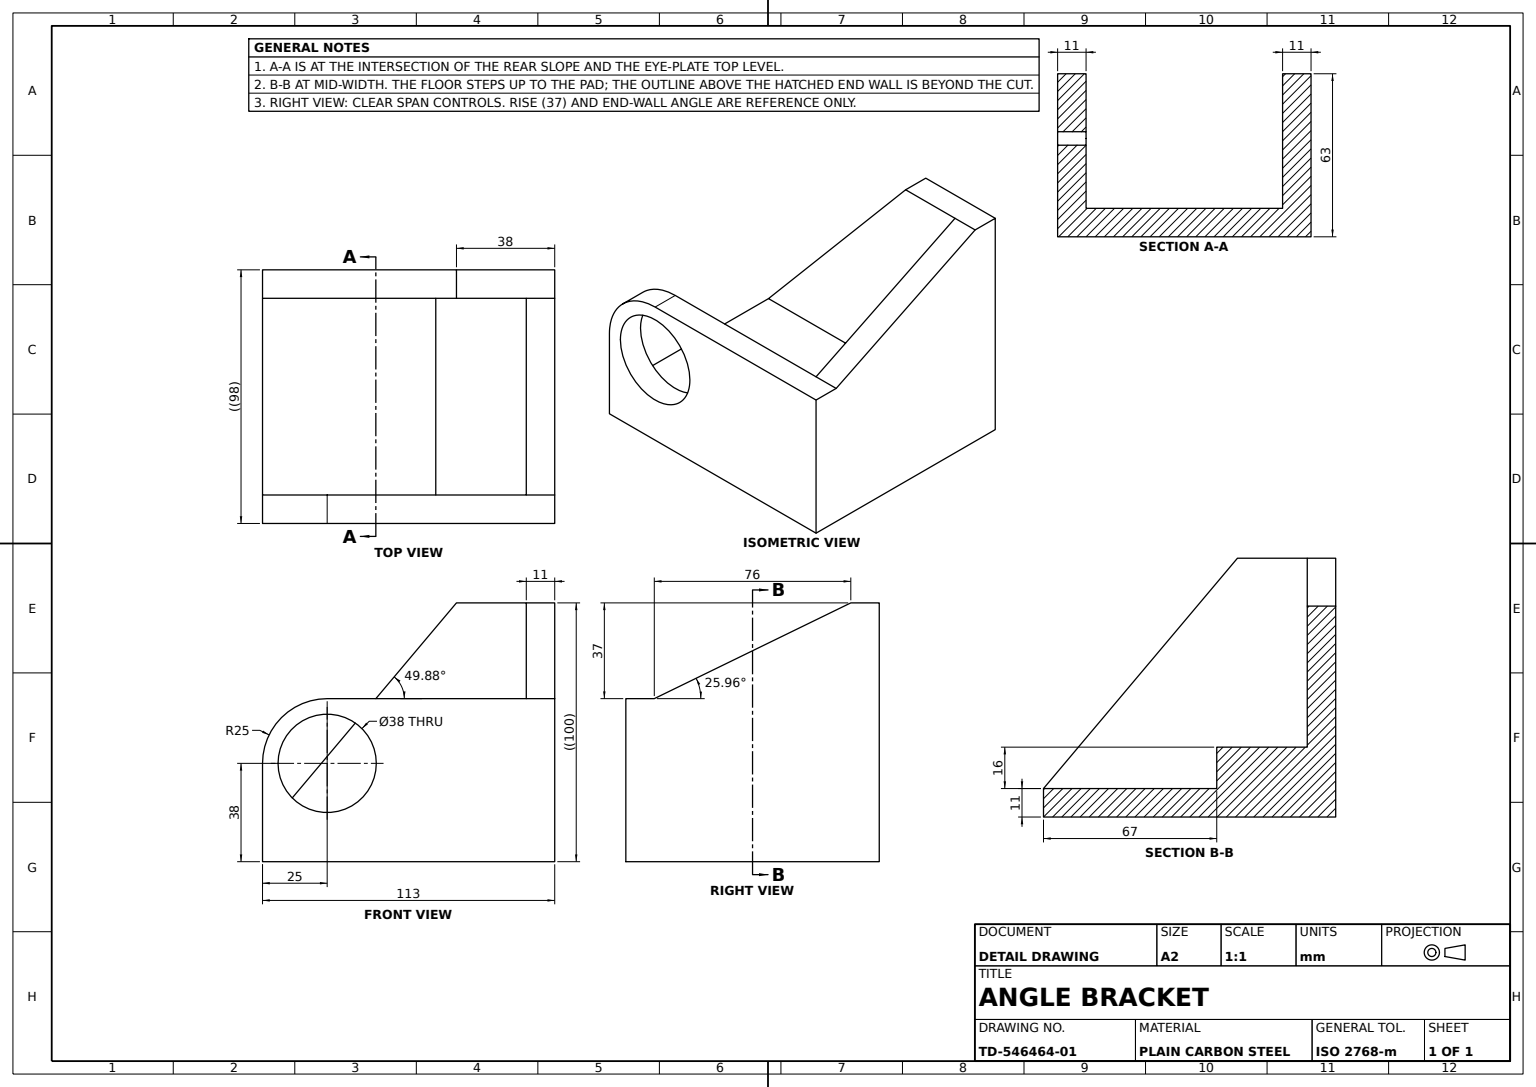
from build123d import *

# Parameters (mm, degrees)
EYE_PLATE_11MM_DEPTH    = 11
FLOOR_PLATE_11MM_DEPTH  = 11
SIDE_WALL_11MM_DEPTH    = 11
INCLINED_WEB_PROFILE_W  = 102
INCLINED_WEB_PROFILE_H  = 76
INCLINED_WEB_11MM_DEPTH = 11
END_CAP_PROFILE_W       = 35
END_CAP_PROFILE_H       = 76
END_CAP_16MM_DEPTH      = 16
PIVOT_BORE_PROFILE_R    = 19
PIVOT_BORE_38_DEPTH     = 11


with BuildPart() as part:
    # Eye Plate Profile → Eye Plate 11mm (new body)
    with BuildSketch(Plane.XY):
        with BuildLine():
            Line((0, 0), (113, 0))
            Line((113, 0), (113, 63))
            Line((113, 63), (25, 63))
            ThreePointArc((25, 63), (7.32233047, 55.67766953), (0, 38))
            Line((0, 38), (0, 0))
        make_face()
    extrude(amount=EYE_PLATE_11MM_DEPTH)

    # Floor Plate Profile → Floor Plate 11mm (add)
    with BuildSketch(Plane(origin=(113, 0, 0), x_dir=(0, 0, -1), z_dir=(1, 0, 0))):
        Polygon((0, 0), (76, 0), (76, 100), (0, 63), align=None)
    extrude(amount=-FLOOR_PLATE_11MM_DEPTH)

    # Side Wall Profile → Side Wall 11mm (add)
    with BuildSketch(Plane(origin=(0, 0, -76), x_dir=(-1, 0, 0), z_dir=(0, 0, -1))):
        Polygon((-113, 0), (0, 0), (0, 11), (-75, 100), (-113, 100), align=None)
    extrude(amount=SIDE_WALL_11MM_DEPTH)

    # Inclined Web Profile → Inclined Web 11mm (add)
    with BuildSketch(Plane.XZ):
        with Locations((51, -38)):
            Rectangle(INCLINED_WEB_PROFILE_W, INCLINED_WEB_PROFILE_H)
    extrude(amount=-INCLINED_WEB_11MM_DEPTH)

    # End Cap Profile → End Cap 16mm (add)
    with BuildSketch(Plane(origin=(0, 11, 0), x_dir=(1, 0, 0), z_dir=(0, 1, 0))):
        with Locations((84.5, 38)):
            Rectangle(END_CAP_PROFILE_W, END_CAP_PROFILE_H)
    extrude(amount=END_CAP_16MM_DEPTH)

    # Pivot Bore Profile → Pivot Bore Ø38 (cut)
    with BuildSketch(Plane.XY.offset(11)):
        with Locations((25, 38)):
            Circle(PIVOT_BORE_PROFILE_R)
    extrude(amount=-PIVOT_BORE_38_DEPTH, mode=Mode.SUBTRACT)


solid = part.part
